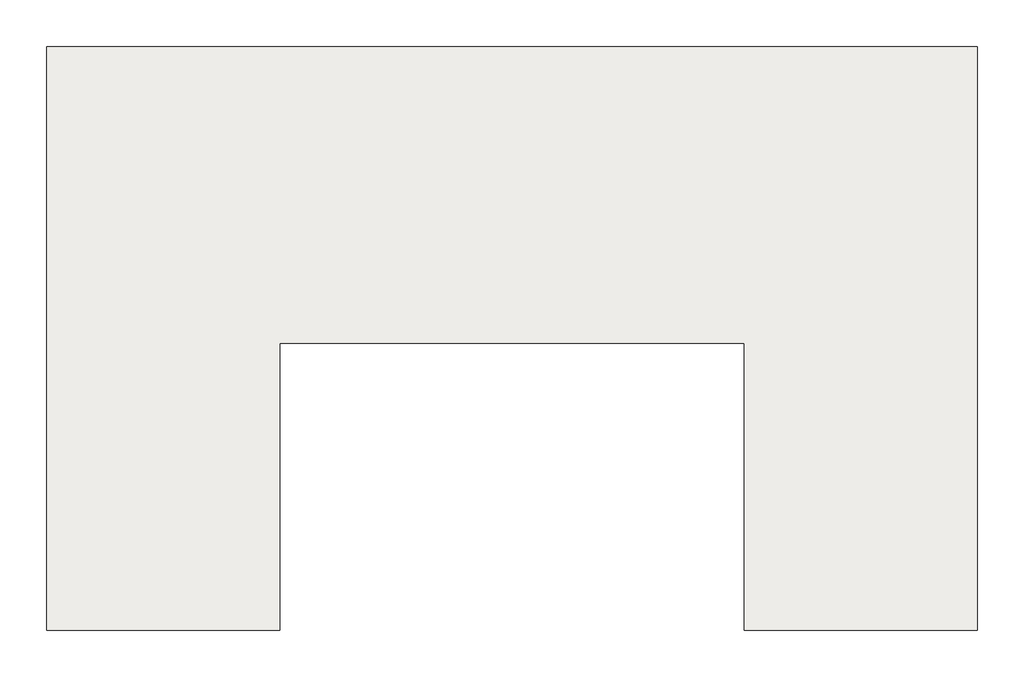
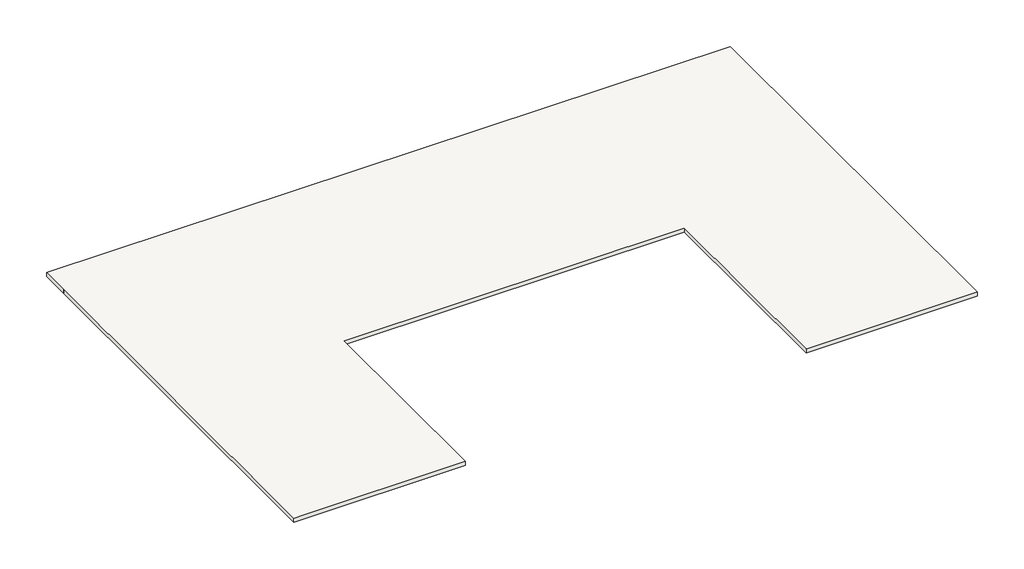
# One storey, part 1 of 2: 1 slab.
"""IFC4 building model written with IfcOpenShell, lengths in millimetres."""

from ifc_helpers import new_model, si_unit, frame, origin, place, context, project, spatial, polyline, outline, extrude, element, save

model = new_model("IFC4")

# Units and contexts
model_context = context("Model", 3, world=origin())
ifc_project = project(units=[si_unit("LENGTHUNIT", "METRE", prefix="MILLI")], contexts=[model_context])

# Site, building, storey
site = spatial("IfcSite", under=ifc_project)
building = spatial("IfcBuilding", under=site)
storey = spatial("IfcBuildingStorey", under=building, Elevation=-2000.0)

# Slab
placement = place(None, origin())
element("IfcSlab", 1, ObjectType="Generic 300mm", at=placement, inside=storey, context=model_context, shape_type="SweptSolid", body=[
    extrude(outline(polyline([(22079.1673137, 16584.1704288), (22079.1673137, -13495.8295712), (10049.1673137, -13495.8295712), (10049.1673137, 1299.0255511), (-13870.8326863, 1299.0255511), (-13870.8326863, -13495.8295712), (-25900.8326863, -13495.8295712), (-25900.8326863, 16584.1704288), (22079.1673137, 16584.1704288)])), frame((0.0, 0.0, -2300.0), z_axis=(0.0, 0.0, 1.0), x_axis=(1.0, 0.0, 0.0)), (0.0, 0.0, 1.0), 300.0),
])

save(model, "model.ifc")

# Revit data of these elements
# Type "Generic 300mm"
#   Function = 0
#   Layers, outside or top first: 300 mm no material (function 1)
# Element 1 (IfcSlab, "Generic 300mm")
#   Height Offset From Level = 0 mm
#   built-in parameter 1001954 = 1
#   Phase Created = New Construction
#   Materials on its faces: "Default Floor"
# Materials
#   "Default Floor": colour RGB 127 127 127, transparency 0, Cost = 0
